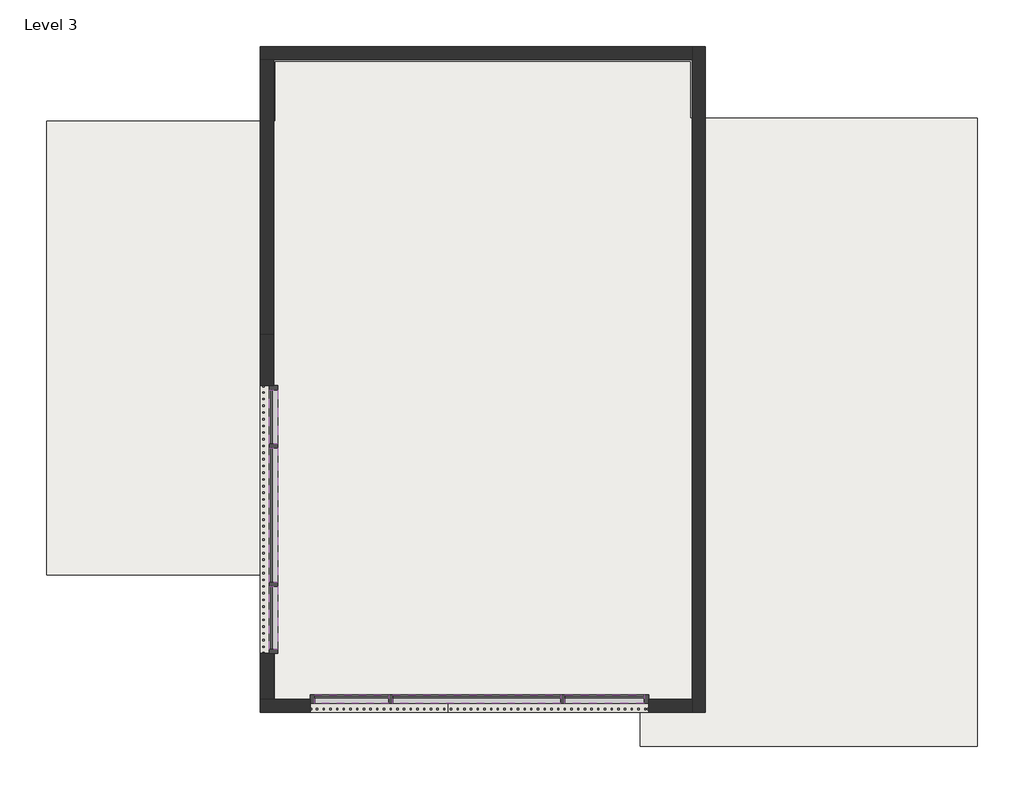
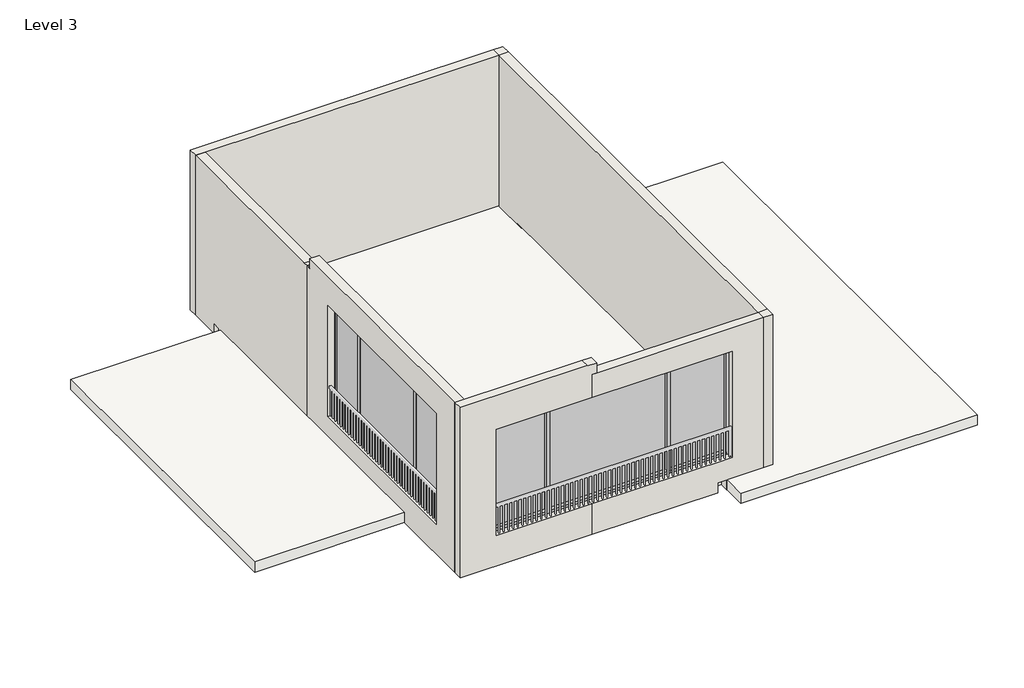
# One storey, part 1 of 2: 20 members, 6 plates, 6 walls, 1 roof.
"""IFC4 building model written with IfcOpenShell, lengths in millimetres."""

from ifc_helpers import new_model, si_unit, frame, origin, place, context, project, spatial, polyline, outline, extrude, faceted_brep, transform, mapped, element, save
from components import member_f0fea5a5, member_ee409385, member_2dd96db1, member_e6b9f524, member_74da8ab1, member_57aae9a7, member_003cbd34, member_c17f1be2, member_bc34c253, member_2b3b556d, system_panel_glazed_5d90cfdf, system_panel_glazed_1974f2ce, system_panel_glazed_4219beb1, system_panel_glazed_5a718088, system_panel_glazed_bafc467c, system_panel_glazed_2306c2a7

model = new_model("IFC4")

# Units and contexts
model_context = context("Model", 3, world=origin())
ifc_project = project(units=[si_unit("LENGTHUNIT", "METRE", prefix="MILLI")], contexts=[model_context])

# Site, building, storey
site = spatial("IfcSite", under=ifc_project)
building = spatial("IfcBuilding", under=site)
storey = spatial("IfcBuildingStorey", under=building, Name="Level 3", Elevation=7315.2)

# Members
placement = place(None, origin())
member_shape = member_f0fea5a5(model_context)
element("IfcMember", 1, ObjectType="Rectangular Mullion : 2.5\" x 5\" rectangular", at=placement, inside=storey, context=model_context, shape_type="MappedRepresentation", body=[
    mapped(member_shape, transform((-10652.0372956, -2089.5372168, 8008.9262316), x_axis=(1.0, 0.0, 0.0), y_axis=(0.0, -1.0, 0.0), z_axis=(0.0, 0.0, -1.0))),
])
element("IfcMember", 2, ObjectType="Rectangular Mullion : 2.5\" x 5\" rectangular", at=placement, inside=storey, context=model_context, shape_type="MappedRepresentation", body=[
    mapped(member_shape, transform((-8044.3039622, -2089.5372168, 8008.9262316), x_axis=(1.0, 0.0, 0.0), y_axis=(0.0, -1.0, 0.0), z_axis=(0.0, 0.0, -1.0))),
])
member_2_shape = member_ee409385(model_context)
element("IfcMember", 3, ObjectType="Rectangular Mullion : 2.5\" x 5\" rectangular", at=placement, inside=storey, context=model_context, shape_type="MappedRepresentation", body=[
    mapped(member_2_shape, transform((-6740.4372956, -2089.5372168, 8008.9262316), x_axis=(1.0, 0.0, 0.0), y_axis=(0.0, -1.0, 0.0), z_axis=(0.0, 0.0, -1.0))),
])
element("IfcMember", 4, ObjectType="Rectangular Mullion : 2.5\" x 5\" rectangular", at=placement, inside=storey, context=model_context, shape_type="MappedRepresentation", body=[
    mapped(member_2_shape, transform((-11871.2372956, -2089.5372168, 10447.3262316), x_axis=(-1.0, 0.0, 0.0), y_axis=(0.0, -1.0, 0.0), z_axis=(0.0, 0.0, 1.0))),
])
member_3_shape = member_2dd96db1(model_context)
element("IfcMember", 5, ObjectType="Rectangular Mullion : 2.5\" x 5\" rectangular", at=placement, inside=storey, context=model_context, shape_type="MappedRepresentation", body=[
    mapped(member_3_shape, transform((-8076.0539622, -2089.5372168, 10447.3262316), x_axis=(0.0, 0.0, 1.0), y_axis=(0.0, -1.0, 0.0), z_axis=(1.0, 0.0, 0.0))),
])
element("IfcMember", 6, ObjectType="Rectangular Mullion : 2.5\" x 5\" rectangular", at=placement, inside=storey, context=model_context, shape_type="MappedRepresentation", body=[
    mapped(member_3_shape, transform((-10620.2872956, -2089.5372168, 8008.9262316), x_axis=(0.0, 0.0, -1.0), y_axis=(0.0, -1.0, 0.0), z_axis=(-1.0, 0.0, 0.0))),
])
member_4_shape = member_e6b9f524(model_context)
element("IfcMember", 7, ObjectType="Rectangular Mullion : 2.5\" x 5\" rectangular", at=placement, inside=storey, context=model_context, shape_type="MappedRepresentation", body=[
    mapped(member_4_shape, transform((-10683.7872956, -2089.5372168, 10447.3262316), x_axis=(0.0, 0.0, 1.0), y_axis=(0.0, -1.0, 0.0), z_axis=(1.0, 0.0, 0.0))),
])
element("IfcMember", 8, ObjectType="Rectangular Mullion : 2.5\" x 5\" rectangular", at=placement, inside=storey, context=model_context, shape_type="MappedRepresentation", body=[
    mapped(member_4_shape, transform((-11807.7372956, -2089.5372168, 8008.9262316), x_axis=(0.0, 0.0, -1.0), y_axis=(0.0, -1.0, 0.0), z_axis=(-1.0, 0.0, 0.0))),
])
member_5_shape = member_74da8ab1(model_context)
element("IfcMember", 9, ObjectType="Rectangular Mullion : 2.5\" x 5\" rectangular", at=placement, inside=storey, context=model_context, shape_type="MappedRepresentation", body=[
    mapped(member_5_shape, transform((-6803.9372956, -2089.5372168, 10447.3262316), x_axis=(0.0, 0.0, 1.0), y_axis=(0.0, -1.0, 0.0), z_axis=(1.0, 0.0, 0.0))),
])
element("IfcMember", 10, ObjectType="Rectangular Mullion : 2.5\" x 5\" rectangular", at=placement, inside=storey, context=model_context, shape_type="MappedRepresentation", body=[
    mapped(member_5_shape, transform((-8012.5539622, -2089.5372168, 8008.9262316), x_axis=(0.0, 0.0, -1.0), y_axis=(0.0, -1.0, 0.0), z_axis=(-1.0, 0.0, 0.0))),
])
member_6_shape = member_57aae9a7(model_context)
element("IfcMember", 11, ObjectType="Rectangular Mullion : 2.5\" x 5\" rectangular", at=placement, inside=storey, context=model_context, shape_type="MappedRepresentation", body=[
    mapped(member_6_shape, transform((-12430.0372956, -378.3217143, 10537.7660302), x_axis=(0.0, 0.0, 1.0), y_axis=(1.0, 0.0, 0.0), z_axis=(0.0, 1.0, 0.0))),
])
member_7_shape = member_003cbd34(model_context)
element("IfcMember", 12, ObjectType="Rectangular Mullion : 2.5\" x 5\" rectangular", at=placement, inside=storey, context=model_context, shape_type="MappedRepresentation", body=[
    mapped(member_7_shape, transform((-12430.0372956, 1721.411619, 10537.7660302), x_axis=(0.0, 0.0, 1.0), y_axis=(1.0, 0.0, 0.0), z_axis=(0.0, 1.0, 0.0))),
])
member_8_shape = member_c17f1be2(model_context)
element("IfcMember", 13, ObjectType="Rectangular Mullion : 2.5\" x 5\" rectangular", at=placement, inside=storey, context=model_context, shape_type="MappedRepresentation", body=[
    mapped(member_8_shape, transform((-12430.0372956, 2604.061619, 10537.7660302), x_axis=(0.0, 0.0, 1.0), y_axis=(1.0, 0.0, 0.0), z_axis=(0.0, 1.0, 0.0))),
])
member_9_shape = member_bc34c253(model_context)
element("IfcMember", 14, ObjectType="Rectangular Mullion : 2.5\" x 5\" rectangular", at=placement, inside=storey, context=model_context, shape_type="MappedRepresentation", body=[
    mapped(member_9_shape, transform((-12430.0372956, -346.5717143, 7997.7660302), x_axis=(0.0, 1.0, 0.0), y_axis=(1.0, 0.0, 0.0), z_axis=(0.0, 0.0, -1.0))),
])
element("IfcMember", 15, ObjectType="Rectangular Mullion : 2.5\" x 5\" rectangular", at=placement, inside=storey, context=model_context, shape_type="MappedRepresentation", body=[
    mapped(member_9_shape, transform((-12430.0372956, 1753.161619, 7997.7660302), x_axis=(0.0, 1.0, 0.0), y_axis=(1.0, 0.0, 0.0), z_axis=(0.0, 0.0, -1.0))),
])
element("IfcMember", 16, ObjectType="Rectangular Mullion : 2.5\" x 5\" rectangular", at=placement, inside=storey, context=model_context, shape_type="MappedRepresentation", body=[
    mapped(member_7_shape, transform((-12430.0372956, -314.8217143, 7997.7660302), x_axis=(0.0, 0.0, -1.0), y_axis=(1.0, 0.0, 0.0), z_axis=(0.0, -1.0, 0.0))),
])
element("IfcMember", 17, ObjectType="Rectangular Mullion : 2.5\" x 5\" rectangular", at=placement, inside=storey, context=model_context, shape_type="MappedRepresentation", body=[
    mapped(member_8_shape, transform((-12430.0372956, 1784.911619, 7997.7660302), x_axis=(0.0, 0.0, -1.0), y_axis=(1.0, 0.0, 0.0), z_axis=(0.0, -1.0, 0.0))),
])
element("IfcMember", 18, ObjectType="Rectangular Mullion : 2.5\" x 5\" rectangular", at=placement, inside=storey, context=model_context, shape_type="MappedRepresentation", body=[
    mapped(member_6_shape, transform((-12430.0372956, -1332.938381, 7997.7660302), x_axis=(0.0, 0.0, -1.0), y_axis=(1.0, 0.0, 0.0), z_axis=(0.0, -1.0, 0.0))),
])
member_10_shape = member_2b3b556d(model_context)
element("IfcMember", 19, ObjectType="Rectangular Mullion : 2.5\" x 5\" rectangular", at=placement, inside=storey, context=model_context, shape_type="MappedRepresentation", body=[
    mapped(member_10_shape, transform((-12430.0372956, -1396.438381, 10537.7660302), x_axis=(0.0, -1.0, 0.0), y_axis=(1.0, 0.0, 0.0), z_axis=(0.0, 0.0, 1.0))),
])
element("IfcMember", 20, ObjectType="Rectangular Mullion : 2.5\" x 5\" rectangular", at=placement, inside=storey, context=model_context, shape_type="MappedRepresentation", body=[
    mapped(member_10_shape, transform((-12430.0372956, 2667.561619, 7997.7660302), x_axis=(0.0, 1.0, 0.0), y_axis=(1.0, 0.0, 0.0), z_axis=(0.0, 0.0, -1.0))),
])

# Plates
system_panel_glazed_shape = system_panel_glazed_5d90cfdf(model_context)
element("IfcPlate", 21, ObjectType="System Panel : Glazed", at=placement, inside=storey, context=model_context, shape_type="MappedRepresentation", body=[
    mapped(system_panel_glazed_shape, transform((-9348.1706289, -2089.5372168, 8072.4262316), x_axis=(1.0, 0.0, 0.0), y_axis=(0.0, 1.0, 0.0), z_axis=(0.0, 0.0, 1.0))),
])
system_panel_glazed_2_shape = system_panel_glazed_1974f2ce(model_context)
element("IfcPlate", 22, ObjectType="System Panel : Glazed", at=placement, inside=storey, context=model_context, shape_type="MappedRepresentation", body=[
    mapped(system_panel_glazed_2_shape, transform((-11245.7622956, -2089.5372168, 8072.4262316), x_axis=(1.0, 0.0, 0.0), y_axis=(0.0, 1.0, 0.0), z_axis=(0.0, 0.0, 1.0))),
])
system_panel_glazed_3_shape = system_panel_glazed_4219beb1(model_context)
element("IfcPlate", 23, ObjectType="System Panel : Glazed", at=placement, inside=storey, context=model_context, shape_type="MappedRepresentation", body=[
    mapped(system_panel_glazed_3_shape, transform((-7408.2456289, -2089.5372168, 8072.4262316), x_axis=(1.0, 0.0, 0.0), y_axis=(0.0, 1.0, 0.0), z_axis=(0.0, 0.0, 1.0))),
])
system_panel_glazed_4_shape = system_panel_glazed_5a718088(model_context)
element("IfcPlate", 24, ObjectType="System Panel : Glazed", at=placement, inside=storey, context=model_context, shape_type="MappedRepresentation", body=[
    mapped(system_panel_glazed_4_shape, transform((-12430.0372956, -855.6300477, 8061.2660302), x_axis=(0.0, 1.0, 0.0), y_axis=(-1.0, 0.0, 0.0), z_axis=(0.0, 0.0, 1.0))),
])
system_panel_glazed_5_shape = system_panel_glazed_bafc467c(model_context)
element("IfcPlate", 25, ObjectType="System Panel : Glazed", at=placement, inside=storey, context=model_context, shape_type="MappedRepresentation", body=[
    mapped(system_panel_glazed_5_shape, transform((-12430.0372956, 2194.486619, 8061.2660302), x_axis=(0.0, 1.0, 0.0), y_axis=(-1.0, 0.0, 0.0), z_axis=(0.0, 0.0, 1.0))),
])
system_panel_glazed_6_shape = system_panel_glazed_2306c2a7(model_context)
element("IfcPlate", 26, ObjectType="System Panel : Glazed", at=placement, inside=storey, context=model_context, shape_type="MappedRepresentation", body=[
    mapped(system_panel_glazed_6_shape, transform((-12430.0372956, 703.2949523, 8061.2660302), x_axis=(0.0, 1.0, 0.0), y_axis=(-1.0, 0.0, 0.0), z_axis=(0.0, 0.0, 1.0))),
])

# Roof
element("IfcRoof", 27, ObjectType="Generic - 9\"", at=placement, inside=storey, context=model_context, shape_type="SweptSolid", body=[
    extrude(outline(polyline([(-15873.211895, -202.638381), (-15873.211895, 6680.761619), (-12404.6372956, 6680.761619), (-12404.6372956, 7587.8627832), (-6105.4372956, 7587.8627832), (-6105.4372956, 6731.561619), (-2792.211895, 6731.561619), (-1750.811895, 6731.561619), (-1750.811895, -2806.138381), (-6868.911895, -2806.138381), (-6868.911895, -2089.5372168), (-12410.9872956, -2089.5372168), (-12410.9872956, -202.638381), (-15873.211895, -202.638381)])), frame((0.0, 0.0, 7315.2), z_axis=(0.0, 0.0, 1.0), x_axis=(1.0, 0.0, 0.0)), (0.0, 0.0, 1.0), 228.6),
])

# Walls
element("IfcWall", 28, ObjectType="Generic - 8\"", at=placement, inside=storey, context=model_context, shape_type="Brep", body=[
    faceted_brep([(-12633.2372956, 7613.2627832, 7315.2), (-12430.0372956, 7613.2627832, 7315.2), (-6080.0372956, 7613.2627832, 7315.2), (-6080.0372956, 7613.2627832, 10972.8), (-12430.0372956, 7613.2627832, 10972.8), (-12633.2372956, 7613.2627832, 10972.8), (-12633.2372956, 7816.4627832, 7315.2), (-12633.2372956, 7816.4627832, 10972.8), (-6080.0372956, 7816.4627832, 10972.8), (-6080.0372956, 7816.4627832, 7315.2)], [[[0, 1, 2, 3, 4, 5]], [[6, 7, 8, 9]], [[2, 1, 0, 6, 9]], [[5, 4, 3, 8, 7]], [[0, 5, 7, 6]], [[3, 2, 9, 8]]]),
])
element("IfcWall", 29, ObjectType="Generic - 8\"", at=placement, inside=storey, context=model_context, shape_type="SweptSolid", body=[
    extrude(outline(polyline([(3447.6627832, 7315.2), (3447.6627832, 10972.8), (3549.2627832, 10972.8), (7613.2627832, 10972.8), (7613.2627832, 7315.2), (6947.8125844, 7315.2), (6947.8125844, 7543.8), (6744.6125844, 7543.8), (6744.6125844, 7315.2), (3447.6627832, 7315.2)])), frame((-12633.2372956, 0.0, 0.0), z_axis=(1.0, 0.0, 0.0), x_axis=(0.0, 1.0, 0.0)), (0.0, 0.0, 1.0), 203.2),
])
element("IfcWall", 30, ObjectType="Generic - 8\"", at=placement, inside=storey, context=model_context, shape_type="Brep", body=[
    faceted_brep([(-6080.0372956, 7816.4627832, 10972.8), (-6080.0372956, 7816.4627832, 7315.2), (-6080.0372956, 7613.2627832, 7315.2), (-6080.0372956, 6947.8125844, 7315.2), (-6080.0372956, 6947.8125844, 7543.8), (-6080.0372956, 6744.6125844, 7543.8), (-6080.0372956, 6744.6125844, 7315.2), (-6080.0372956, -2089.5372168, 7315.2), (-6080.0372956, -2292.7372168, 7315.2), (-6080.0372956, -2292.7372168, 10972.8), (-6080.0372956, -2089.5372168, 10972.8), (-6080.0372956, 7613.2627832, 10972.8), (-5876.8372956, 7816.4627832, 7315.2), (-5876.8372956, 7816.4627832, 10972.8), (-5876.8372956, 7613.2627832, 10972.8), (-5876.8372956, -2089.5372168, 10972.8), (-5876.8372956, -2292.7372168, 10972.8), (-5876.8372956, -2292.7372168, 7315.2), (-5876.8372956, 6744.6125844, 7315.2), (-5876.8372956, 6744.6125844, 7543.8), (-5876.8372956, 6947.8125844, 7543.8), (-5876.8372956, 6947.8125844, 7315.2)], [[[0, 1, 2, 3, 4, 5, 6, 7, 8, 9, 10, 11]], [[12, 13, 14, 15, 16, 17, 18, 19, 20, 21]], [[1, 12, 21, 3, 2]], [[17, 8, 7, 6, 18]], [[1, 0, 13, 12]], [[13, 0, 11, 14]], [[10, 9, 16, 15]], [[14, 11, 10, 15]], [[9, 8, 17, 16]], [[5, 19, 18, 6]], [[20, 4, 3, 21]], [[19, 5, 4, 20]]]),
])
element("IfcWall", 31, ObjectType="Generic - 8\"", at=placement, inside=storey, context=model_context, shape_type="Brep", body=[
    faceted_brep([(-12633.2372956, -2292.7372168, 7315.2), (-9788.4372956, -2292.7372168, 7315.2), (-9788.4372956, -2292.7372168, 8008.9262316), (-11871.2372956, -2292.7372168, 8008.9262316), (-11871.2372956, -2292.7372168, 10447.3262316), (-9890.0372956, -2292.7372168, 10447.3262316), (-9788.4372956, -2292.7372168, 10447.3262316), (-9788.4372956, -2292.7372168, 10972.8), (-9686.8372956, -2292.7372168, 10972.8), (-9686.8372956, -2292.7372168, 11201.4), (-9890.0372956, -2292.7372168, 11201.4), (-9890.0372956, -2292.7372168, 11209.3262316), (-12633.2372956, -2292.7372168, 11209.3262316), (-12633.2372956, -2089.5372168, 7315.2), (-12633.2372956, -2089.5372168, 11201.4), (-12633.2372956, -2089.5372168, 11209.3262316), (-9890.0372956, -2089.5372168, 11209.3262316), (-9890.0372956, -2089.5372168, 11201.4), (-9686.8372956, -2089.5372168, 11201.4), (-9686.8372956, -2089.5372168, 10972.8), (-9788.4372956, -2089.5372168, 10972.8), (-9788.4372956, -2089.5372168, 10447.3262316), (-9890.0372956, -2089.5372168, 10447.3262316), (-11871.2372956, -2089.5372168, 10447.3262316), (-11871.2372956, -2089.5372168, 8008.9262316), (-9788.4372956, -2089.5372168, 8008.9262316), (-9788.4372956, -2089.5372168, 7315.2), (-12430.0372956, -2089.5372168, 7315.2)], [[[0, 1, 2, 3, 4, 5, 6, 7, 8, 9, 10, 11, 12]], [[13, 14, 15, 16, 17, 18, 19, 20, 21, 22, 23, 24, 25, 26, 27]], [[0, 12, 15, 14, 13]], [[1, 0, 13, 27, 26]], [[12, 11, 16, 15]], [[2, 1, 26, 25]], [[3, 2, 25, 24]], [[4, 3, 24, 23]], [[5, 4, 23, 22]], [[6, 5, 22, 21]], [[7, 6, 21, 20]], [[19, 8, 7, 20]], [[17, 10, 9, 18]], [[8, 19, 18, 9]], [[11, 10, 17, 16]]]),
])
element("IfcWall", 32, ObjectType="Generic - 8\"", at=placement, inside=storey, context=model_context, shape_type="Brep", body=[
    faceted_brep([(-6080.0372956, -2292.7372168, 10972.8), (-9686.8372956, -2292.7372168, 10972.8), (-9788.4372956, -2292.7372168, 10972.8), (-9788.4372956, -2292.7372168, 10447.3262316), (-6740.4372956, -2292.7372168, 10447.3262316), (-6740.4372956, -2292.7372168, 8008.9262316), (-9788.4372956, -2292.7372168, 8008.9262316), (-9788.4372956, -2292.7372168, 7315.2), (-7073.4141623, -2292.7372168, 7315.2), (-7073.4141623, -2292.7372168, 7541.577893), (-6870.2141623, -2292.7372168, 7541.577893), (-6870.2141623, -2292.7372168, 7315.2), (-6080.0372956, -2292.7372168, 7315.2), (-9788.4372956, -2089.5372168, 10972.8), (-9686.8372956, -2089.5372168, 10972.8), (-6080.0372956, -2089.5372168, 10972.8), (-6080.0372956, -2089.5372168, 7315.2), (-6870.2141623, -2089.5372168, 7315.2), (-6870.2141623, -2089.5372168, 7541.577893), (-7073.4141623, -2089.5372168, 7541.577893), (-7073.4141623, -2089.5372168, 7315.2), (-9788.4372956, -2089.5372168, 7315.2), (-9788.4372956, -2089.5372168, 8008.9262316), (-6740.4372956, -2089.5372168, 8008.9262316), (-6740.4372956, -2089.5372168, 10447.3262316), (-9788.4372956, -2089.5372168, 10447.3262316)], [[[0, 1, 2, 3, 4, 5, 6, 7, 8, 9, 10, 11, 12]], [[13, 14, 15, 16, 17, 18, 19, 20, 21, 22, 23, 24, 25]], [[0, 12, 16, 15]], [[19, 9, 8, 20]], [[10, 18, 17, 11]], [[9, 19, 18, 10]], [[16, 12, 11, 17]], [[7, 21, 20, 8]], [[2, 1, 0, 15, 14, 13]], [[3, 2, 13, 25]], [[4, 3, 25, 24]], [[5, 4, 24, 23]], [[6, 5, 23, 22]], [[7, 6, 22, 21]]]),
])
element("IfcWall", 33, ObjectType="Generic - 8\"", at=placement, inside=storey, context=model_context, shape_type="Brep", body=[
    faceted_brep([(-12633.2372956, 3447.6627832, 7315.2), (-12633.2372956, -214.9874156, 7315.2), (-12633.2372956, -418.1874156, 7315.2), (-12633.2372956, -2089.5372168, 7315.2), (-12633.2372956, -2089.5372168, 11201.4), (-12633.2372956, 3346.0627832, 11201.4), (-12633.2372956, 3346.0627832, 10972.8), (-12633.2372956, 3447.6627832, 10972.8), (-12633.2372956, -1396.438381, 10537.7660302), (-12633.2372956, -1396.438381, 7997.7660302), (-12633.2372956, 2667.561619, 7997.7660302), (-12633.2372956, 2667.561619, 10537.7660302), (-12430.0372956, 3447.6627832, 7315.2), (-12430.0372956, 3447.6627832, 10972.8), (-12430.0372956, 3346.0627832, 10972.8), (-12430.0372956, 3346.0627832, 11201.4), (-12430.0372956, -2089.5372168, 11201.4), (-12430.0372956, -2089.5372168, 7315.2), (-12430.0372956, -1396.438381, 10537.7660302), (-12430.0372956, 2667.561619, 10537.7660302), (-12430.0372956, 2667.561619, 7997.7660302), (-12430.0372956, -1396.438381, 7997.7660302)], [[[0, 1, 2, 3, 4, 5, 6, 7], [8, 9, 10, 11]], [[12, 13, 14, 15, 16, 17], [18, 19, 20, 21]], [[6, 5, 15, 14]], [[4, 3, 17, 16]], [[3, 2, 1, 0, 12, 17]], [[5, 4, 16, 15]], [[0, 7, 13, 12]], [[6, 14, 13, 7]], [[9, 8, 18, 21]], [[10, 9, 21, 20]], [[11, 10, 20, 19]], [[8, 11, 19, 18]]]),
])

save(model, "model.ifc")

# Revit data of these elements
# Type "Rectangular Mullion : 2.5\" x 5\" rectangular"
#   built-in parameter 1007304 = 0.416667 (stored number, unit not read)
#   built-in parameter 1007301 = 0.104167 (stored number, unit not read)
#   built-in parameter 1007300 = 0.104167 (stored number, unit not read)
# Type "System Panel : Glazed"
#   Construction Type Id = "GSP4R"
#   Analytic Construction = "1/8 in Pilkington single glazing"
#   Visual Light Transmittance = 0.9
#   Solar Heat Gain Coefficient = 0.86
#   Heat Transfer Coefficient (U) = 1.18115 BTU/(h·ft²·°F)
# Type "Generic - 9\""
#   Assembly Code = "B1020"
#   Layers, outside or top first: 0' - 9" no material (function 1)
# Type "Generic - 8\""
#   Assembly Code = "B2010"
#   Layers, outside or top first: 0' - 8" no material (function 1)
# Elements 1, 2, 3, 4, 5, 6, 7, 8, 9, 10, 11, 12, 13, 14, 15, 16, 17, 18, 19, 20 (IfcMember, "Rectangular Mullion : 2.5\" x 5\" rectangular")
#   Phase Created = New Construction
#   Materials on its faces: "Aluminum"
# Elements 21, 22, 23, 24, 25, 26 (IfcPlate, "System Panel : Glazed")
#   Phase Created = New Construction
#   Materials on its faces: "Glass"
# Element 27 (IfcRoof, "Generic - 9\"")
#   built-in parameter 1001705 = 24.75 (stored number, unit not read)
#   built-in parameter 1001710 = 33615
#   Phase Created = New Construction
#   Materials on its faces: "Default Roof", "Cherry"
# Elements 28, 29, 32 (IfcWall, "Generic - 8\"")
#   Top Offset = 0' - 0"
#   Base Offset = 0' - 0"
#   Unconnected Height = 12' - 0"
#   wall height = 12' - 0"
#   Phase Created = New Construction
#   Base Constraint = Level 3
#   Materials on its faces: "Default Wall", "Gypsum Wall Board"
# Element 30 (IfcWall, "Generic - 8\"")
#   Top Offset = 0' - 0"
#   Base Offset = 0' - 0"
#   Unconnected Height = 12' - 0"
#   wall height = 12' - 0"
#   Phase Created = New Construction
#   Base Constraint = Level 3
#   Materials on its faces: "Default Wall", "Cherry", "Gypsum Wall Board"
# Element 31 (IfcWall, "Generic - 8\"")
#   Top Offset = 0' - 0"
#   Base Offset = 0' - 0"
#   Unconnected Height = 12' - 9.31206"
#   wall height = 12' - 9.31206"
#   Phase Created = New Construction
#   Base Constraint = Level 3
#   Materials on its faces: "Default Wall", "Gypsum Wall Board"
# Element 33 (IfcWall, "Generic - 8\"")
#   Top Offset = 0' - 0"
#   Base Offset = 0' - 0"
#   Unconnected Height = 12' - 9"
#   wall height = 12' - 9"
#   Phase Created = New Construction
#   Base Constraint = Level 3
#   Materials on its faces: "Default Wall", "Gypsum Wall Board"
# Materials
#   "Aluminum": class "Metal", colour RGB 247 247 247, transparency 0, Description = "Aluminum 6061", Cost = 0
#   "Glass": class "Glass", colour RGB 0 128 192, transparency 0.75, Description = "Soda Lime Glass", Cost = 0
#   "Default Roof": colour RGB 88 101 114, transparency 0
#   "Cherry": class "Wood", colour RGB 226 177 128, transparency 0, Description = "Prunus Serotina", Cost = 0
#   "Default Wall": colour RGB 128 128 128, transparency 0
#   "Gypsum Wall Board": class "Generic", colour RGB 127 127 127, transparency 0, Description = "Gypsum Wall Board", Cost = 0
